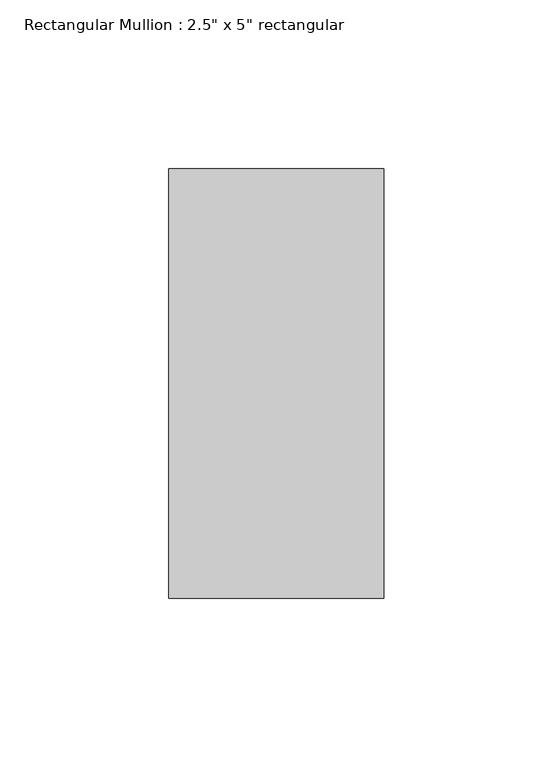
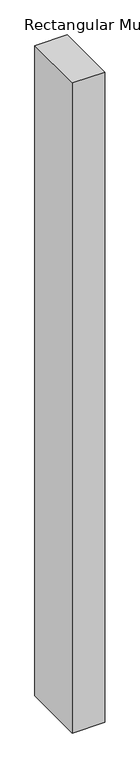
"""IFC4 building model written with IfcOpenShell, lengths in millimetres: member geometry."""

from ifc_helpers import new_model, si_unit, frame, origin, place, context, project, spatial, polyline, outline, extrude, source, transform, mapped, element, save


def member_05f3a264(model_context):
    return source(origin(), model_context, "Body", "SweptSolid", [
        extrude(outline(polyline([(31.75, 63.5), (31.75, -63.5), (-31.75, -63.5), (-31.75, 63.5), (31.75, 63.5)])), frame((0.0, 0.0, -1347.9161516), z_axis=(0.0, 0.0, 1.0), x_axis=(1.0, 0.0, 0.0)), (0.0, 0.0, 1.0), 1347.9161516),
    ])


if __name__ == "__main__":
    model = new_model("IFC4")
    model_context = context("Model", 3, world=origin())
    ifc_project = project(units=[si_unit("LENGTHUNIT", "METRE", prefix="MILLI")], contexts=[model_context])
    site = spatial("IfcSite", under=ifc_project)
    building = spatial("IfcBuilding", under=site)
    placement = place(None, origin())
    member_shape = member_05f3a264(model_context)
    element("IfcMember", 1, ObjectType="Rectangular Mullion : 2.5\" x 5\" rectangular", at=placement, inside=building, context=model_context, shape_type="MappedRepresentation", body=[
        mapped(member_shape, transform((0.0, 0.0, 0.0), x_axis=(1.0, 0.0, 0.0), y_axis=(0.0, 1.0, 0.0), z_axis=(0.0, 0.0, 1.0))),
    ])
    save(model, "model.ifc")

# Revit data of these elements
# Type "Rectangular Mullion : 2.5\" x 5\" rectangular"
#   built-in parameter 1007304 = 0.416667 (stored number, unit not read)
#   built-in parameter 1007301 = 0.104167 (stored number, unit not read)
#   built-in parameter 1007300 = 0.104167 (stored number, unit not read)
# Element 1 (IfcMember, "Rectangular Mullion : 2.5\" x 5\" rectangular")
#   Materials on its faces: "Aluminum"
# Materials
#   "Aluminum": class "Metal", colour RGB 247 247 247, transparency 0, Description = "Aluminum 6061", Cost = 0
